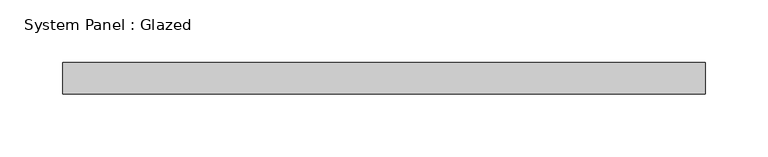
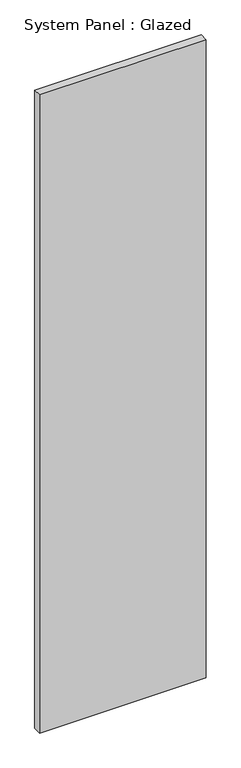
"""IFC4 building model written with IfcOpenShell, lengths in millimetres: plate geometry, System Panel : Glazed."""

from ifc_helpers import new_model, si_unit, origin, origin_with_axes, place, context, project, spatial, polyline, outline, extrude, source, transform, mapped, element, save


def system_panel_glazed_e322ed92(model_context):
    return source(origin(), model_context, "Body", "SweptSolid", [
        extrude(outline(polyline([(257.175, 19.05), (-257.175, 19.05), (-257.175, 44.45), (257.175, 44.45), (257.175, 19.05)])), origin_with_axes(), (0.0, 0.0, 1.0), 2082.8),
    ])


if __name__ == "__main__":
    model = new_model("IFC4")
    model_context = context("Model", 3, world=origin())
    ifc_project = project(units=[si_unit("LENGTHUNIT", "METRE", prefix="MILLI")], contexts=[model_context])
    site = spatial("IfcSite", under=ifc_project)
    building = spatial("IfcBuilding", under=site)
    placement = place(None, origin())
    system_panel_glazed_shape = system_panel_glazed_e322ed92(model_context)
    element("IfcPlate", 1, ObjectType="System Panel : Glazed", at=placement, inside=building, context=model_context, shape_type="MappedRepresentation", body=[
        mapped(system_panel_glazed_shape, transform((0.0, 0.0, 0.0), x_axis=(1.0, 0.0, 0.0), y_axis=(0.0, 1.0, 0.0), z_axis=(0.0, 0.0, 1.0))),
    ])
    save(model, "model.ifc")

# Revit data of these elements
# Type "System Panel : Glazed"
#   Construction Type Id = "GSP4R"
#   Analytic Construction = "1/8 in Pilkington single glazing"
#   Visual Light Transmittance = 0.9
#   Solar Heat Gain Coefficient = 0.86
#   Heat Transfer Coefficient (U) = 1.18115 BTU/(h·ft²·°F)
#   Define Thermal Properties by = 1
# Element 1 (IfcPlate, "System Panel : Glazed")
#   Materials on its faces: "Glass"
# Materials
#   "Glass": class "Glass", colour RGB 0 128 192, transparency 0.75, Description = "Soda Lime Glass", Cost = 0
